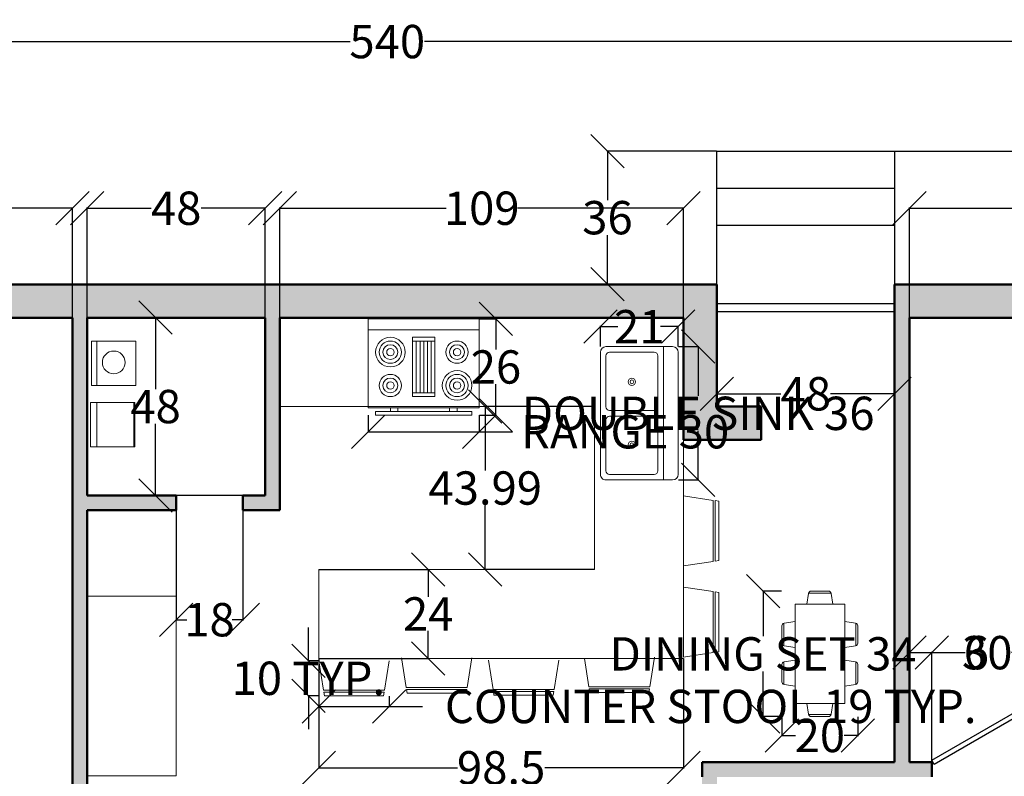
# Model space of a CAD drawing. Units: inches. Extents: x -9 to 615, y -420 to 89.
# Tile 5 of 6: x 201 to 467, y -115 to 89. Entities that reach past the tile are written whole.
import ezdxf

# ---------------------------------------------------------------- set-up
doc = ezdxf.new("R2010")
doc.units = ezdxf.units.IN
doc.header["$MEASUREMENT"] = 0
for name, color, linetype, lineweight in [('A-ANNO-DIMS', 2, 'Continuous', 18), ('A-DOOR', 4, 'Continuous', 25), ('A-EQPM', 8, 'Continuous', 18), ('A-FLOR-CASE', 32, 'Continuous', 18), ('A-FLOR-FIXT', 9, 'Continuous', 18), ('A-FLOR-STRS', 7, 'Continuous', 25), ('A-FURN', 8, 'Continuous', 18), ('A-WALL', 7, 'Continuous', 50)]:
    doc.layers.add(name, color=color, linetype=linetype, lineweight=lineweight)
doc.layers.add('A-WALL-PATT', color=251, linetype='Continuous', lineweight=13, true_color=0x636466)
doc.styles.get("Standard").update_dxf_attribs({"font": 'arial.ttf'})
doc.dimstyles.get("Standard").update_dxf_attribs({"dimtxt": 9, "dimasz": 9, "dimexe": 0.18, "dimexo": 0.0625, "dimgap": 0.09, "dimtad": 0, "dimtih": 1, "dimtoh": 1, "dimdec": 0, "dimzin": 0, "dimdsep": 46, "dimlunit": 4, "dimtxsty": 'Standard', "dimblk": 'OBLIQUE', "dimblk2": 'OBLIQUE', "dimcen": 0.09, "dimadec": 0, "dimazin": 0, "dimtfac": 1, "dimtdec": 0, "dimtofl": 0, "dimtmove": 0, "dimatfit": 3, "dimldrblk": 'OBLIQUE', "dimfxl": 1, "dimtolj": 1, "dimtzin": 0, "dimarcsym": 0})

# ---------------------------------------------------------------- blocks, each defined once
blk = doc.blocks.new('Range-Oven - 30 in top')
for p, q in [((0, -3), (30, -3)), ((12, -6), (18, -6)), ((13, -20), (13, -6)), ((14, -6), (14, -20)), ((15, -20), (15, -6)), ((16, -6), (16, -20)), ((17, -20), (17, -6)), ((18, -20), (12, -20)), ((6, -24), (6, -25)), ((8, -25), (8, -24)), ((22, -25), (22, -24)), ((24, -24), (24, -25))]:
    blk.add_line(p, q)
for points in [[(0, -24), (0, 0), (30, 0), (30, -24)], [(12, -21), (12, -5), (18, -5), (18, -21)], [(2, -26), (2, -25), (28, -25), (28, -26)]]:
    blk.add_lwpolyline(points, close=True)
for centre, radius in [((6, -9), 4), ((6, -9), 3), ((6, -9), 2), ((24, -9), 3), ((24, -9), 2), ((6, -9), 1), ((24, -9), 1), ((6, -18), 3), ((24, -18), 4), ((24, -18), 3), ((6, -18), 2), ((6, -18), 1), ((24, -18), 2), ((24, -18), 1)]:
    blk.add_circle(centre, radius)
blk = doc.blocks.new('Sink-double - 36 in top')
for p, q in [((-18, -4), (18, -4)), ((-0.75, -18.5), (-0.75, -6.5)), ((0.75, -6.5), (0.75, -18.5))]:
    blk.add_line(p, q)
for points in [[(-16.5, 0), (16.5, 0)], [(-18, -19.5), (-18, -1.5)], [(18, -1.5), (18, -19.5)], [(-16.5, -18.5), (-16.5, -6.5)], [(-15.5, -5.5), (-1.75, -5.5)], [(1.75, -5.5), (15.5, -5.5)], [(16.5, -6.5), (16.5, -18.5)], [(16.5, -21), (-16.5, -21)], [(-1.75, -19.5), (-15.5, -19.5)], [(15.5, -19.5), (1.75, -19.5)]]:
    blk.add_lwpolyline(points)
for centre, radius in [((-8.5, -12.5), 1), ((-8.5, -12.5), 0.5), ((8.5, -12.5), 1), ((8.5, -12.5), 0.5)]:
    blk.add_circle(centre, radius)
for centre, radius, start, end in [((-16.5, -1.5), 1.5, 90, 180), ((16.5, -1.5), 1.5, 0, 90), ((-15.5, -6.5), 1, 90, 180), ((-1.75, -6.5), 1, 0, 90), ((1.75, -6.5), 1, 90, 180), ((15.5, -6.5), 1, 0, 90), ((-15.5, -18.5), 1, 180, 270), ((-1.75, -18.5), 1, 270, 0), ((1.75, -18.5), 1, 180, 270), ((15.5, -18.5), 1, 270, 0), ((-16.5, -19.5), 1.5, 180, 270), ((16.5, -19.5), 1.5, 270, 0)]:
    blk.add_arc(centre, radius, start, end)
blk = doc.blocks.new('Dining Set - 36 x 72 in.')
for p, q in [((-22.26, 25.81), (-23.48, 18)), ((-22.23, 26), (-5.76, 26)), ((-20.29, 27.5), (-7.71, 27.5)), ((-4.52, 18), (-5.74, 25.81)), ((5.74, 25.81), (4.52, 18)), ((5.77, 26), (22.24, 26)), ((7.71, 27.5), (20.29, 27.5)), ((23.48, 18), (22.26, 25.81)), ((36, 18), (-36, 18)), ((-36, 18), (-36, -18)), ((36, -18), (36, 18)), ((-44, 8.23), (-44, -8.24)), ((-43.81, 8.26), (-36, 9.48)), ((43.81, 8.26), (36, 9.48)), ((44, 8.23), (44, -8.24)), ((-45.5, 6.29), (-45.5, -6.29)), ((45.5, 6.29), (45.5, -6.29)), ((-36, -9.48), (-43.81, -8.26)), ((36, -9.48), (43.81, -8.26)), ((-36, -18), (36, -18)), ((-22.26, -25.81), (-23.48, -18)), ((-4.52, -18), (-5.74, -25.81)), ((5.74, -25.81), (4.52, -18)), ((23.48, -18), (22.26, -25.81)), ((-22.23, -26), (-5.76, -26)), ((-20.29, -27.5), (-7.71, -27.5)), ((5.77, -26), (22.24, -26)), ((7.71, -27.5), (20.29, -27.5))]:
    blk.add_line(p, q)
for centre, start, end in [((-20.29, 25.5), 90, 171.11979), ((-7.71, 25.5), 8.88096, 90), ((7.71, 25.5), 90, 171.11979), ((20.29, 25.5), 8.88096, 90), ((-43.5, 6.29), 98.8806, 180), ((43.5, 6.29), 0, 81.1194), ((-43.5, -6.29), 180, 261.11938), ((43.5, -6.29), 278.88062, 0), ((-20.29, -25.5), 188.8802, 270), ((-7.71, -25.5), 270, 351.11906), ((7.71, -25.5), 188.8802, 270), ((20.29, -25.5), 270, 351.11906)]:
    blk.add_arc(centre, 2, start, end)
blk = doc.blocks.new('*U14')
for p, q in [((0, 0), (0, 6)), ((40, 0), (40, 6))]:
    blk.add_line(p, q)
blk.add_lwpolyline([(0, 0), (40, 0), (40, 1.75), (0, 1.75)], close=True)
blk = doc.blocks.new('*U12')
for p, q in [((0, 0), (0, -6)), ((40, 0), (40, -6))]:
    blk.add_line(p, q)
blk.add_lwpolyline([(0, 0), (34.64, 20), (35.52, 18.48), (0.87, -1.52)], close=True)
blk.add_arc((0, 0), 40, 0, 30)
blk = doc.blocks.new('CHAIR-COUNTER')
for p, q in [((8, 17.72), (0, 18.97)), ((8, 17.72), (8, 1.25)), ((9.5, 17.48), (8.5, 17.64)), ((8.5, 1.33), (8.5, 17.64)), ((9.5, 17.48), (9.5, 1.48)), ((0, 0), (8, 1.25)), ((8.5, 1.33), (9.5, 1.48))]:
    blk.add_line(p, q)
blk = doc.blocks.new('_Oblique')
at = {"color": 0, "linetype": 'ByBlock', "lineweight": -2}
blk.add_line((-0.5, -0.5), (0.5, 0.5), dxfattribs=at)
blk = doc.blocks.new('*D26')
at = {"layer": 'A-ANNO-DIMS', "color": 0, "lineweight": -2, "transparency": 16777216}
for p, q in [((281.97, -93.16), (281.97, -96.13)), ((300.94, -93.16), (300.94, -96.13)), ((281.97, -95.95), (300.94, -95.95)), ((300.94, -95.95), (309.94, -95.95))]:
    blk.add_line(p, q, dxfattribs=at)
at = {"layer": 'Defpoints', "color": 0, "transparency": 16777216}
for p in [(281.97, -93.1), (300.94, -93.1), (300.94, -95.95)]:
    blk.add_point(p, dxfattribs=at)
at = {"layer": 'A-ANNO-DIMS', "color": 0, "lineweight": -2, "transparency": 16777216, "xscale": 9, "yscale": 9, "zscale": 9, "rotation": 180}
blk.add_blockref('_Oblique', (281.97, -95.95), dxfattribs=at)
at = {"layer": 'A-ANNO-DIMS', "color": 0, "lineweight": -2, "transparency": 16777216, "xscale": 9, "yscale": 9, "zscale": 9}
blk.add_blockref('_Oblique', (300.94, -95.95), dxfattribs=at)
at = {"layer": 'A-ANNO-DIMS', "color": 0, "transparency": 16777216, "insert": (387.77, -95.95), "char_height": 9, "attachment_point": 5}
blk.add_mtext('\\A1;COUNTER STOOL 19 TYP.', dxfattribs=at)
blk = doc.blocks.new('*D27')
at = {"layer": 'A-ANNO-DIMS', "color": 0, "lineweight": -2, "transparency": 16777216}
for p, q in [((279.13, -83.6), (279.13, -74.6)), ((281.91, -83.6), (278.95, -83.6)), ((281.91, -93.1), (278.95, -93.1)), ((279.13, -93.1), (279.13, -102.1))]:
    blk.add_line(p, q, dxfattribs=at)
at = {"layer": 'Defpoints', "color": 0, "transparency": 16777216}
for p in [(281.97, -83.6), (279.13, -93.1), (281.97, -93.1)]:
    blk.add_point(p, dxfattribs=at)
at = {"layer": 'A-ANNO-DIMS', "color": 0, "lineweight": -2, "transparency": 16777216, "xscale": 9, "yscale": 9, "zscale": 9}
for p, rotation in [((279.13, -83.6), 270), ((279.13, -93.1), 90)]:
    blk.add_blockref('_Oblique', p, dxfattribs=dict(at, rotation=rotation))
at = {"layer": 'A-ANNO-DIMS', "color": 0, "transparency": 16777216, "insert": (279.13, -88.35), "char_height": 9, "attachment_point": 5}
blk.add_mtext('\\A1;10 TYP.', dxfattribs=at)
blk = doc.blocks.new('*D32')
at = {"layer": 'A-ANNO-DIMS', "color": 0, "lineweight": -2, "transparency": 16777216}
for p, q in [((295.28, -17.35), (295.28, -21.97)), ((325.28, -17.35), (325.28, -21.97)), ((295.28, -21.79), (325.28, -21.79)), ((325.28, -21.79), (334.28, -21.79))]:
    blk.add_line(p, q, dxfattribs=at)
at = {"layer": 'Defpoints', "color": 0, "transparency": 16777216}
for p in [(295.28, -17.29), (325.28, -17.29), (325.28, -21.79)]:
    blk.add_point(p, dxfattribs=at)
at = {"layer": 'A-ANNO-DIMS', "color": 0, "lineweight": -2, "transparency": 16777216, "xscale": 9, "yscale": 9, "zscale": 9, "rotation": 180}
blk.add_blockref('_Oblique', (295.28, -21.79), dxfattribs=at)
at = {"layer": 'A-ANNO-DIMS', "color": 0, "lineweight": -2, "transparency": 16777216, "xscale": 9, "yscale": 9, "zscale": 9}
blk.add_blockref('_Oblique', (325.28, -21.79), dxfattribs=at)
at = {"layer": 'A-ANNO-DIMS', "color": 0, "transparency": 16777216, "insert": (364.67, -21.79), "char_height": 9, "attachment_point": 5}
blk.add_mtext('\\A1;RANGE 30', dxfattribs=at)
blk = doc.blocks.new('*D33')
at = {"layer": 'A-ANNO-DIMS', "color": 0, "lineweight": -2, "transparency": 16777216}
for p, q in [((325.34, 8.71), (329.96, 8.71)), ((329.78, 8.71), (329.78, 0.4)), ((329.78, -17.29), (329.78, -8.97)), ((325.34, -17.29), (329.96, -17.29))]:
    blk.add_line(p, q, dxfattribs=at)
at = {"layer": 'Defpoints', "color": 0, "transparency": 16777216}
for p in [(325.28, 8.71), (329.78, 8.71), (325.28, -17.29)]:
    blk.add_point(p, dxfattribs=at)
at = {"layer": 'A-ANNO-DIMS', "color": 0, "lineweight": -2, "transparency": 16777216, "xscale": 9, "yscale": 9, "zscale": 9}
for p, rotation in [((329.78, 8.71), 90), ((329.78, -17.29), 270)]:
    blk.add_blockref('_Oblique', p, dxfattribs=dict(at, rotation=rotation))
at = {"layer": 'A-ANNO-DIMS', "color": 0, "transparency": 16777216, "insert": (329.78, -4.29), "char_height": 9, "attachment_point": 5}
blk.add_mtext('\\A1;26', dxfattribs=at)
blk = doc.blocks.new('*D34')
at = {"layer": 'A-ANNO-DIMS', "color": 0, "lineweight": -2, "transparency": 16777216}
for p, q in [((379.05, 1.19), (384.57, 1.19)), ((384.39, 1.19), (384.39, -12.06)), ((384.39, -34.81), (384.39, -21.56)), ((379.05, -34.81), (384.57, -34.81))]:
    blk.add_line(p, q, dxfattribs=at)
at = {"layer": 'Defpoints', "color": 0, "transparency": 16777216}
for p in [(378.99, 1.19), (378.99, -34.81), (384.39, -34.81)]:
    blk.add_point(p, dxfattribs=at)
at = {"layer": 'A-ANNO-DIMS', "color": 0, "lineweight": -2, "transparency": 16777216, "xscale": 9, "yscale": 9, "zscale": 9}
for p, rotation in [((384.39, 1.19), 90), ((384.39, -34.81), 270)]:
    blk.add_blockref('_Oblique', p, dxfattribs=dict(at, rotation=rotation))
at = {"layer": 'A-ANNO-DIMS', "color": 0, "transparency": 16777216, "insert": (384.39, -16.81), "char_height": 9, "attachment_point": 5}
blk.add_mtext('\\A1;DOUBLE SINK 36', dxfattribs=at)
blk = doc.blocks.new('*D35')
at = {"layer": 'A-ANNO-DIMS', "color": 0, "lineweight": -2, "transparency": 16777216}
for p, q in [((357.99, 1.25), (357.99, 6.77)), ((357.99, 6.59), (362.74, 6.59)), ((378.99, 6.59), (374.23, 6.59)), ((378.99, 1.25), (378.99, 6.77))]:
    blk.add_line(p, q, dxfattribs=at)
at = {"layer": 'Defpoints', "color": 0, "transparency": 16777216}
for p in [(378.99, 6.59), (357.99, 1.19), (378.99, 1.19)]:
    blk.add_point(p, dxfattribs=at)
at = {"layer": 'A-ANNO-DIMS', "color": 0, "lineweight": -2, "transparency": 16777216, "xscale": 9, "yscale": 9, "zscale": 9, "rotation": 180}
blk.add_blockref('_Oblique', (357.99, 6.59), dxfattribs=at)
at = {"layer": 'A-ANNO-DIMS', "color": 0, "lineweight": -2, "transparency": 16777216, "xscale": 9, "yscale": 9, "zscale": 9}
blk.add_blockref('_Oblique', (378.99, 6.59), dxfattribs=at)
at = {"layer": 'A-ANNO-DIMS', "color": 0, "transparency": 16777216, "insert": (368.49, 6.59), "char_height": 9, "attachment_point": 5}
blk.add_mtext('\\A1;21', dxfattribs=at)
blk = doc.blocks.new('*D38')
at = {"layer": 'A-ANNO-DIMS', "color": 0, "lineweight": -2, "transparency": 16777216}
for p, q in [((406.93, -64.79), (401.73, -64.79)), ((401.91, -64.79), (401.91, -77)), ((401.91, -98.71), (401.91, -86.5)), ((406.93, -98.71), (401.73, -98.71))]:
    blk.add_line(p, q, dxfattribs=at)
at = {"layer": 'Defpoints', "color": 0, "transparency": 16777216}
for p in [(407, -64.79), (401.91, -98.71), (407, -98.71)]:
    blk.add_point(p, dxfattribs=at)
at = {"layer": 'A-ANNO-DIMS', "color": 0, "lineweight": -2, "transparency": 16777216, "xscale": 9, "yscale": 9, "zscale": 9}
for p, rotation in [((401.91, -64.79), 90), ((401.91, -98.71), 270)]:
    blk.add_blockref('_Oblique', p, dxfattribs=dict(at, rotation=rotation))
at = {"layer": 'A-ANNO-DIMS', "color": 0, "transparency": 16777216, "insert": (401.91, -81.75), "char_height": 9, "attachment_point": 5}
blk.add_mtext('\\A1;DINING SET 34', dxfattribs=at)
blk = doc.blocks.new('*D39')
at = {"layer": 'A-ANNO-DIMS', "color": 0, "lineweight": -2, "transparency": 16777216}
for p, q in [((407, -98.77), (407, -103.97)), ((427.49, -98.77), (427.49, -103.97)), ((407, -103.79), (410.65, -103.79)), ((427.49, -103.79), (423.84, -103.79))]:
    blk.add_line(p, q, dxfattribs=at)
at = {"layer": 'Defpoints', "color": 0, "transparency": 16777216}
for p in [(407, -98.71), (427.49, -98.71), (427.49, -103.79)]:
    blk.add_point(p, dxfattribs=at)
at = {"layer": 'A-ANNO-DIMS', "color": 0, "lineweight": -2, "transparency": 16777216, "xscale": 9, "yscale": 9, "zscale": 9, "rotation": 180}
blk.add_blockref('_Oblique', (407, -103.79), dxfattribs=at)
at = {"layer": 'A-ANNO-DIMS', "color": 0, "lineweight": -2, "transparency": 16777216, "xscale": 9, "yscale": 9, "zscale": 9}
blk.add_blockref('_Oblique', (427.49, -103.79), dxfattribs=at)
at = {"layer": 'A-ANNO-DIMS', "color": 0, "transparency": 16777216, "insert": (417.24, -103.79), "char_height": 9, "attachment_point": 5}
blk.add_mtext('\\A1;20', dxfattribs=at)
blk = doc.blocks.new('*D40')
at = {"layer": 'A-ANNO-DIMS', "color": 0, "lineweight": -2, "transparency": 16777216}
for p, q in [((30.44, 18.08), (30.44, 83.75)), ((30.44, 83.57), (290.42, 83.57)), ((570.44, 83.57), (310.45, 83.57)), ((570.44, 18.08), (570.44, 83.75))]:
    blk.add_line(p, q, dxfattribs=at)
at = {"layer": 'Defpoints', "color": 0, "transparency": 16777216}
for p in [(570.44, 83.57), (30.44, 18.02), (570.44, 18.02)]:
    blk.add_point(p, dxfattribs=at)
at = {"layer": 'A-ANNO-DIMS', "color": 0, "lineweight": -2, "transparency": 16777216, "xscale": 9, "yscale": 9, "zscale": 9, "rotation": 180}
blk.add_blockref('_Oblique', (30.44, 83.57), dxfattribs=at)
at = {"layer": 'A-ANNO-DIMS', "color": 0, "lineweight": -2, "transparency": 16777216, "xscale": 9, "yscale": 9, "zscale": 9}
blk.add_blockref('_Oblique', (570.44, 83.57), dxfattribs=at)
at = {"layer": 'A-ANNO-DIMS', "color": 0, "transparency": 16777216, "insert": (300.44, 83.57), "char_height": 9, "attachment_point": 5}
blk.add_mtext('\\A1;540', dxfattribs=at)
blk = doc.blocks.new('*D42')
at = {"layer": 'A-ANNO-DIMS', "color": 0, "lineweight": -2, "transparency": 16777216}
for p, q in [((437.5, 54.02), (600.17, 54.02)), ((599.99, 54.02), (599.99, -160.45)), ((599.99, -384.29), (599.99, -169.82)), ((365.62, -384.29), (600.17, -384.29))]:
    blk.add_line(p, q, dxfattribs=at)
at = {"layer": 'Defpoints', "color": 0, "transparency": 16777216}
for p in [(437.44, 54.02), (599.99, 54.02), (365.56, -384.29)]:
    blk.add_point(p, dxfattribs=at)
at = {"layer": 'A-ANNO-DIMS', "color": 0, "lineweight": -2, "transparency": 16777216, "xscale": 9, "yscale": 9, "zscale": 9}
for p, rotation in [((599.99, 54.02), 90), ((599.99, -384.29), 270)]:
    blk.add_blockref('_Oblique', p, dxfattribs=dict(at, rotation=rotation))
at = {"layer": 'A-ANNO-DIMS', "color": 0, "transparency": 16777216, "insert": (599.99, -165.14), "char_height": 9, "attachment_point": 5}
blk.add_mtext('\\A1;438.3', dxfattribs=at)
blk = doc.blocks.new('*D43')
at = {"layer": 'A-ANNO-DIMS', "color": 0, "lineweight": -2, "transparency": 16777216}
for p, q in [((39.44, 9.08), (39.44, 38.75)), ((39.44, 38.57), (117.83, 38.57)), ((215.44, 38.57), (137.04, 38.57)), ((215.44, 9.08), (215.44, 38.75))]:
    blk.add_line(p, q, dxfattribs=at)
at = {"layer": 'Defpoints', "color": 0, "transparency": 16777216}
for p in [(215.44, 38.57), (39.44, 9.02), (215.44, 9.02)]:
    blk.add_point(p, dxfattribs=at)
at = {"layer": 'A-ANNO-DIMS', "color": 0, "lineweight": -2, "transparency": 16777216, "xscale": 9, "yscale": 9, "zscale": 9, "rotation": 180}
blk.add_blockref('_Oblique', (39.44, 38.57), dxfattribs=at)
at = {"layer": 'A-ANNO-DIMS', "color": 0, "lineweight": -2, "transparency": 16777216, "xscale": 9, "yscale": 9, "zscale": 9}
blk.add_blockref('_Oblique', (215.44, 38.57), dxfattribs=at)
at = {"layer": 'A-ANNO-DIMS', "color": 0, "transparency": 16777216, "insert": (127.44, 38.57), "char_height": 9, "attachment_point": 5}
blk.add_mtext('\\A1;176', dxfattribs=at)
blk = doc.blocks.new('*D44')
at = {"layer": 'A-ANNO-DIMS', "color": 0, "lineweight": -2, "transparency": 16777216}
for p, q in [((219.44, 9.08), (219.44, 38.75)), ((219.44, 38.57), (236.71, 38.57)), ((267.44, 38.57), (250.16, 38.57)), ((267.44, 9.08), (267.44, 38.75))]:
    blk.add_line(p, q, dxfattribs=at)
at = {"layer": 'Defpoints', "color": 0, "transparency": 16777216}
for p in [(267.44, 38.57), (219.44, 9.02), (267.44, 9.02)]:
    blk.add_point(p, dxfattribs=at)
at = {"layer": 'A-ANNO-DIMS', "color": 0, "lineweight": -2, "transparency": 16777216, "xscale": 9, "yscale": 9, "zscale": 9, "rotation": 180}
blk.add_blockref('_Oblique', (219.44, 38.57), dxfattribs=at)
at = {"layer": 'A-ANNO-DIMS', "color": 0, "lineweight": -2, "transparency": 16777216, "xscale": 9, "yscale": 9, "zscale": 9}
blk.add_blockref('_Oblique', (267.44, 38.57), dxfattribs=at)
at = {"layer": 'A-ANNO-DIMS', "color": 0, "transparency": 16777216, "insert": (243.44, 38.57), "char_height": 9, "attachment_point": 5}
blk.add_mtext('\\A1;48', dxfattribs=at)
blk = doc.blocks.new('*D45')
at = {"layer": 'A-ANNO-DIMS', "color": 0, "lineweight": -2, "transparency": 16777216}
for p, q in [((271.44, 9.08), (271.44, 38.75)), ((271.44, 38.57), (316.32, 38.57)), ((380.44, 38.57), (335.56, 38.57)), ((380.44, 9.08), (380.44, 38.75))]:
    blk.add_line(p, q, dxfattribs=at)
at = {"layer": 'Defpoints', "color": 0, "transparency": 16777216}
for p in [(380.44, 38.57), (271.44, 9.02), (380.44, 9.02)]:
    blk.add_point(p, dxfattribs=at)
at = {"layer": 'A-ANNO-DIMS', "color": 0, "lineweight": -2, "transparency": 16777216, "xscale": 9, "yscale": 9, "zscale": 9, "rotation": 180}
blk.add_blockref('_Oblique', (271.44, 38.57), dxfattribs=at)
at = {"layer": 'A-ANNO-DIMS', "color": 0, "lineweight": -2, "transparency": 16777216, "xscale": 9, "yscale": 9, "zscale": 9}
blk.add_blockref('_Oblique', (380.44, 38.57), dxfattribs=at)
at = {"layer": 'A-ANNO-DIMS', "color": 0, "transparency": 16777216, "insert": (325.94, 38.57), "char_height": 9, "attachment_point": 5}
blk.add_mtext('\\A1;109', dxfattribs=at)
blk = doc.blocks.new('*D46')
at = {"layer": 'A-ANNO-DIMS', "color": 0, "lineweight": -2, "transparency": 16777216}
for p, q in [((389.44, 17.96), (389.44, -11.71)), ((437.44, 17.96), (437.44, -11.71)), ((389.44, -11.53), (406.71, -11.53)), ((437.44, -11.53), (420.16, -11.53))]:
    blk.add_line(p, q, dxfattribs=at)
at = {"layer": 'Defpoints', "color": 0, "transparency": 16777216}
for p in [(389.44, 18.02), (437.44, 18.02), (389.44, -11.53)]:
    blk.add_point(p, dxfattribs=at)
at = {"layer": 'A-ANNO-DIMS', "color": 0, "lineweight": -2, "transparency": 16777216, "xscale": 9, "yscale": 9, "zscale": 9, "rotation": 180}
blk.add_blockref('_Oblique', (389.44, -11.53), dxfattribs=at)
at = {"layer": 'A-ANNO-DIMS', "color": 0, "lineweight": -2, "transparency": 16777216, "xscale": 9, "yscale": 9, "zscale": 9}
blk.add_blockref('_Oblique', (437.44, -11.53), dxfattribs=at)
at = {"layer": 'A-ANNO-DIMS', "color": 0, "transparency": 16777216, "insert": (413.44, -11.53), "char_height": 9, "attachment_point": 5}
blk.add_mtext('\\A1;48', dxfattribs=at)
blk = doc.blocks.new('*D47')
at = {"layer": 'A-ANNO-DIMS', "color": 0, "lineweight": -2, "transparency": 16777216}
for p, q in [((441.44, 9.08), (441.44, 38.75)), ((441.44, 38.57), (491.84, 38.57)), ((561.44, 38.57), (511.03, 38.57)), ((561.44, 9.08), (561.44, 38.75))]:
    blk.add_line(p, q, dxfattribs=at)
at = {"layer": 'Defpoints', "color": 0, "transparency": 16777216}
for p in [(561.44, 38.57), (441.44, 9.02), (561.44, 9.02)]:
    blk.add_point(p, dxfattribs=at)
at = {"layer": 'A-ANNO-DIMS', "color": 0, "lineweight": -2, "transparency": 16777216, "xscale": 9, "yscale": 9, "zscale": 9, "rotation": 180}
blk.add_blockref('_Oblique', (441.44, 38.57), dxfattribs=at)
at = {"layer": 'A-ANNO-DIMS', "color": 0, "lineweight": -2, "transparency": 16777216, "xscale": 9, "yscale": 9, "zscale": 9}
blk.add_blockref('_Oblique', (561.44, 38.57), dxfattribs=at)
at = {"layer": 'A-ANNO-DIMS', "color": 0, "transparency": 16777216, "insert": (501.44, 38.57), "char_height": 9, "attachment_point": 5}
blk.add_mtext('\\A1;120', dxfattribs=at)
blk = doc.blocks.new('*D48')
at = {"layer": 'A-ANNO-DIMS', "color": 0, "lineweight": -2, "transparency": 16777216}
for p, q in [((389.38, 54.02), (359.71, 54.02)), ((359.89, 54.02), (359.89, 40.71)), ((359.89, 18.02), (359.89, 31.33)), ((389.38, 18.02), (359.71, 18.02))]:
    blk.add_line(p, q, dxfattribs=at)
at = {"layer": 'Defpoints', "color": 0, "transparency": 16777216}
for p in [(359.89, 54.02), (389.44, 54.02), (389.44, 18.02)]:
    blk.add_point(p, dxfattribs=at)
at = {"layer": 'A-ANNO-DIMS', "color": 0, "lineweight": -2, "transparency": 16777216, "xscale": 9, "yscale": 9, "zscale": 9}
for p, rotation in [((359.89, 54.02), 90), ((359.89, 18.02), 270)]:
    blk.add_blockref('_Oblique', p, dxfattribs=dict(at, rotation=rotation))
at = {"layer": 'A-ANNO-DIMS', "color": 0, "transparency": 16777216, "insert": (359.89, 36.02), "char_height": 9, "attachment_point": 5}
blk.add_mtext('\\A1;36', dxfattribs=at)
blk = doc.blocks.new('*D64')
at = {"layer": 'A-ANNO-DIMS', "color": 0, "lineweight": -2, "transparency": 16777216}
for p, q in [((267.38, 9.02), (237.71, 9.02)), ((237.89, 9.02), (237.89, -10.3)), ((237.89, -38.98), (237.89, -19.67)), ((267.38, -38.98), (237.71, -38.98))]:
    blk.add_line(p, q, dxfattribs=at)
at = {"layer": 'Defpoints', "color": 0, "transparency": 16777216}
for p in [(237.89, 9.02), (267.44, 9.02), (267.44, -38.98)]:
    blk.add_point(p, dxfattribs=at)
at = {"layer": 'A-ANNO-DIMS', "color": 0, "lineweight": -2, "transparency": 16777216, "xscale": 9, "yscale": 9, "zscale": 9}
for p, rotation in [((237.89, 9.02), 90), ((237.89, -38.98), 270)]:
    blk.add_blockref('_Oblique', p, dxfattribs=dict(at, rotation=rotation))
at = {"layer": 'A-ANNO-DIMS', "color": 0, "transparency": 16777216, "insert": (237.89, -14.98), "char_height": 9, "attachment_point": 5}
blk.add_mtext('\\A1;48', dxfattribs=at)
blk = doc.blocks.new('*D69')
at = {"layer": 'A-ANNO-DIMS', "color": 0, "lineweight": -2, "transparency": 16777216}
for p, q in [((281.94, -83.03), (281.94, -112.7)), ((380.44, -83.03), (380.44, -112.7)), ((281.94, -112.52), (319.37, -112.52)), ((380.44, -112.52), (343, -112.52))]:
    blk.add_line(p, q, dxfattribs=at)
at = {"layer": 'Defpoints', "color": 0, "transparency": 16777216}
for p in [(281.94, -82.97), (380.44, -82.97), (281.94, -112.52)]:
    blk.add_point(p, dxfattribs=at)
at = {"layer": 'A-ANNO-DIMS', "color": 0, "lineweight": -2, "transparency": 16777216, "xscale": 9, "yscale": 9, "zscale": 9, "rotation": 180}
blk.add_blockref('_Oblique', (281.94, -112.52), dxfattribs=at)
at = {"layer": 'A-ANNO-DIMS', "color": 0, "lineweight": -2, "transparency": 16777216, "xscale": 9, "yscale": 9, "zscale": 9}
blk.add_blockref('_Oblique', (380.44, -112.52), dxfattribs=at)
at = {"layer": 'A-ANNO-DIMS', "color": 0, "transparency": 16777216, "insert": (331.19, -112.52), "char_height": 9, "attachment_point": 5}
blk.add_mtext('\\A1;98.5', dxfattribs=at)
blk = doc.blocks.new('*D70')
at = {"layer": 'A-ANNO-DIMS', "color": 0, "lineweight": -2, "transparency": 16777216}
for p, q in [((356.38, -14.98), (326.71, -14.98)), ((326.89, -14.98), (326.89, -32.29)), ((326.89, -58.97), (326.89, -41.66)), ((356.38, -58.97), (326.71, -58.97))]:
    blk.add_line(p, q, dxfattribs=at)
at = {"layer": 'Defpoints', "color": 0, "transparency": 16777216}
for p in [(326.89, -14.98), (356.44, -14.98), (356.44, -58.97)]:
    blk.add_point(p, dxfattribs=at)
at = {"layer": 'A-ANNO-DIMS', "color": 0, "lineweight": -2, "transparency": 16777216, "xscale": 9, "yscale": 9, "zscale": 9}
for p, rotation in [((326.89, -14.98), 90), ((326.89, -58.97), 270)]:
    blk.add_blockref('_Oblique', p, dxfattribs=dict(at, rotation=rotation))
at = {"layer": 'A-ANNO-DIMS', "color": 0, "transparency": 16777216, "insert": (326.89, -36.98), "char_height": 9, "attachment_point": 5}
blk.add_mtext('\\A1;43.99', dxfattribs=at)
blk = doc.blocks.new('*D71')
at = {"layer": 'A-ANNO-DIMS', "color": 0, "lineweight": -2, "transparency": 16777216}
for p, q in [((282, -58.97), (311.67, -58.97)), ((311.49, -58.97), (311.49, -66.36)), ((311.49, -82.97), (311.49, -75.58)), ((282, -82.97), (311.67, -82.97))]:
    blk.add_line(p, q, dxfattribs=at)
at = {"layer": 'Defpoints', "color": 0, "transparency": 16777216}
for p in [(281.94, -58.97), (281.94, -82.97), (311.49, -82.97)]:
    blk.add_point(p, dxfattribs=at)
at = {"layer": 'A-ANNO-DIMS', "color": 0, "lineweight": -2, "transparency": 16777216, "xscale": 9, "yscale": 9, "zscale": 9}
for p, rotation in [((311.49, -58.97), 90), ((311.49, -82.97), 270)]:
    blk.add_blockref('_Oblique', p, dxfattribs=dict(at, rotation=rotation))
at = {"layer": 'A-ANNO-DIMS', "color": 0, "transparency": 16777216, "insert": (311.49, -70.97), "char_height": 9, "attachment_point": 5}
blk.add_mtext('\\A1;24', dxfattribs=at)
blk = doc.blocks.new('*D81')
at = {"layer": 'A-ANNO-DIMS', "color": 0, "lineweight": -2, "transparency": 16777216}
for p, q in [((441.44, -110.92), (441.44, -81.25)), ((441.44, -81.43), (447.44, -81.43)), ((447.44, -110.92), (447.44, -81.25)), ((447.44, -81.43), (456.44, -81.43))]:
    blk.add_line(p, q, dxfattribs=at)
at = {"layer": 'Defpoints', "color": 0, "transparency": 16777216}
for p in [(447.44, -81.43), (441.44, -110.98), (447.44, -110.98)]:
    blk.add_point(p, dxfattribs=at)
at = {"layer": 'A-ANNO-DIMS', "color": 0, "lineweight": -2, "transparency": 16777216, "xscale": 9, "yscale": 9, "zscale": 9, "rotation": 180}
blk.add_blockref('_Oblique', (441.44, -81.43), dxfattribs=at)
at = {"layer": 'A-ANNO-DIMS', "color": 0, "lineweight": -2, "transparency": 16777216, "xscale": 9, "yscale": 9, "zscale": 9}
blk.add_blockref('_Oblique', (447.44, -81.43), dxfattribs=at)
at = {"layer": 'A-ANNO-DIMS', "color": 0, "transparency": 16777216, "insert": (459.5, -81.43), "char_height": 9, "attachment_point": 5}
blk.add_mtext('\\A1;6', dxfattribs=at)
blk = doc.blocks.new('*D82')
at = {"layer": 'A-ANNO-DIMS', "color": 0, "lineweight": -2, "transparency": 16777216}
for p, q in [((447.44, -110.92), (447.44, -81.25)), ((447.44, -81.43), (455.92, -81.43)), ((477.44, -81.43), (468.96, -81.43)), ((477.44, -110.92), (477.44, -81.25))]:
    blk.add_line(p, q, dxfattribs=at)
at = {"layer": 'Defpoints', "color": 0, "transparency": 16777216}
for p in [(477.44, -81.43), (447.44, -110.98), (477.44, -110.98)]:
    blk.add_point(p, dxfattribs=at)
at = {"layer": 'A-ANNO-DIMS', "color": 0, "lineweight": -2, "transparency": 16777216, "xscale": 9, "yscale": 9, "zscale": 9, "rotation": 180}
blk.add_blockref('_Oblique', (447.44, -81.43), dxfattribs=at)
at = {"layer": 'A-ANNO-DIMS', "color": 0, "lineweight": -2, "transparency": 16777216, "xscale": 9, "yscale": 9, "zscale": 9}
blk.add_blockref('_Oblique', (477.44, -81.43), dxfattribs=at)
at = {"layer": 'A-ANNO-DIMS', "color": 0, "transparency": 16777216, "insert": (462.44, -81.43), "char_height": 9, "attachment_point": 5}
blk.add_mtext('\\A1;30', dxfattribs=at)
blk = doc.blocks.new('*D89')
at = {"layer": 'A-ANNO-DIMS', "color": 0, "lineweight": -2, "transparency": 16777216}
for p, q in [((243.44, -43.04), (243.44, -72.71)), ((261.44, -43.04), (261.44, -72.71)), ((243.44, -72.53), (246.32, -72.53)), ((261.44, -72.53), (258.56, -72.53))]:
    blk.add_line(p, q, dxfattribs=at)
at = {"layer": 'Defpoints', "color": 0, "transparency": 16777216}
for p in [(243.44, -42.98), (261.44, -42.98), (243.44, -72.53)]:
    blk.add_point(p, dxfattribs=at)
at = {"layer": 'A-ANNO-DIMS', "color": 0, "lineweight": -2, "transparency": 16777216, "xscale": 9, "yscale": 9, "zscale": 9, "rotation": 180}
blk.add_blockref('_Oblique', (243.44, -72.53), dxfattribs=at)
at = {"layer": 'A-ANNO-DIMS', "color": 0, "lineweight": -2, "transparency": 16777216, "xscale": 9, "yscale": 9, "zscale": 9}
blk.add_blockref('_Oblique', (261.44, -72.53), dxfattribs=at)
at = {"layer": 'A-ANNO-DIMS', "color": 0, "transparency": 16777216, "insert": (252.44, -72.53), "char_height": 9, "attachment_point": 5}
blk.add_mtext('\\A1;18', dxfattribs=at)

msp = doc.modelspace()

# ---------------------------------------------------------------- hatches: boundary and pattern name
at = {"layer": 'A-WALL-PATT'}
h = msp.add_hatch(color=256, dxfattribs=at)
h.dxf.hatch_style = 1
h.paths.add_polyline_path([(389.4378, 18.0183), (30.4378, 18.0183), (30.4378, -341.9817), (316.4378, -341.9817), (316.4378, -336.5817), (316.4378, -332.9817), (283.4378, -332.9817), (283.4378, -256.9817), (283.4378, -250.9817), (283.4378, -248.9817), (278.9378, -248.9817), (277.4378, -248.9817), (277.4378, -250.9817), (277.4378, -256.9817), (211.4378, -256.9817), (211.4378, -260.9817), (279.4378, -260.9817), (279.4378, -332.9817), (175.4378, -332.9817), (175.4378, -260.9817), (181.4378, -260.9817), (181.4378, -256.9817), (175.4378, -256.9817), (175.4378, -248.9817), (171.4378, -248.9817), (171.4378, -332.9817), (39.4378, -332.9817), (39.4378, -212.9817), (171.4378, -212.9817), (171.4378, -218.9817), (175.4378, -218.9817), (175.4378, -212.9817), (179.4378, -212.9817), (179.4378, -208.9817), (135.4378, -208.9817), (135.4378, -114.9817), (179.4378, -114.9817), (179.4378, -110.9817), (100.4378, -110.9817), (100.4378, -114.9817), (131.4378, -114.9817), (131.4378, -208.9817), (39.4378, -208.9817), (39.4378, -114.9817), (70.4378, -114.9817), (70.4378, -110.9817), (39.4378, -110.9817), (39.4378, 9.0183), (215.4378, 9.0183), (215.4378, -110.9817), (215.4378, -208.9817), (209.4378, -208.9817), (209.4378, -212.9817), (215.4378, -212.9817), (255.4378, -212.9817), (277.4378, -212.9817), (277.4378, -218.9817), (283.4378, -218.9817), (283.4378, -212.9817), (283.4378, -208.9817), (283.4378, -202.9817), (279.4378, -202.9817), (279.4378, -208.9817), (255.4378, -208.9817), (219.4378, -208.9817), (219.4378, -170.1983), (255.4378, -170.1983), (277.4378, -170.1983), (277.4378, -176.1983), (283.4378, -176.1983), (283.4378, -170.1983), (283.4378, -166.1983), (255.4378, -166.1983), (219.4378, -166.1983), (219.4378, -42.9817), (243.4378, -42.9817), (243.4378, -38.9817), (219.4378, -38.9817), (219.4378, 9.0183), (267.4378, 9.0183), (267.4378, -38.9817), (261.4378, -38.9817), (261.4378, -42.9817), (271.4378, -42.9817), (271.4378, 9.0183), (380.4378, 9.0183), (380.4378, -14.9817), (380.4378, -23.9817), (401.4378, -23.9817), (401.4378, -14.9817), (389.4378, -14.9817)])
h = msp.add_hatch(color=256, dxfattribs=at)
h.dxf.hatch_style = 1
h.paths.add_polyline_path([(570.4378, 18.0183), (437.4378, 18.0183), (437.4378, -14.9817), (437.4378, -110.9817), (385.4378, -110.9817), (385.4378, -114.9817), (385.4378, -120.9817), (389.4378, -120.9817), (389.4378, -114.9817), (437.4378, -114.9817), (447.4378, -114.9817), (447.4378, -110.9817), (441.4378, -110.9817), (441.4378, 9.0183), (561.4378, 9.0183), (561.4378, -110.9817), (477.4378, -110.9817), (477.4378, -114.9817), (497.4378, -114.9817), (497.4378, -168.9817), (501.4378, -168.9817), (501.4378, -114.9817), (561.4378, -114.9817), (561.4378, -198.9817), (531.4378, -198.9817), (501.4378, -198.9817), (501.4378, -192.9817), (497.4378, -192.9817), (497.4378, -198.9817), (477.4378, -198.9817), (477.4378, -202.9817), (561.4378, -202.9817), (561.4378, -332.9817), (441.4378, -332.9817), (441.4378, -202.9817), (447.4378, -202.9817), (447.4378, -198.9817), (437.4378, -198.9817), (431.4378, -198.9817), (431.4378, -202.9817), (437.4378, -202.9817), (437.4378, -256.9817), (389.4378, -256.9817), (389.4378, -202.9799), (407.5704, -202.9799), (407.4511, -198.9817), (389.4378, -198.9817), (385.4378, -198.9817), (385.4378, -302.9817), (389.4378, -302.9817), (389.4378, -260.9817), (437.4378, -260.9817), (437.4378, -332.9817), (389.4378, -332.9817), (389.4378, -326.9817), (385.4378, -326.9817), (385.4378, -332.9817), (352.4378, -332.9817), (352.4378, -341.9817), (570.4378, -341.9817)])

# ---------------------------------------------------------------- linework, layer by layer
at = {"layer": 'A-EQPM'}
for p, q in [((221.9973, 2.7027), (221.9973, -9.2973)), ((222.0477, -13.8957), (222.0477, -25.8957)), ((231.9831, -13.8957), (231.9831, -25.8957))]:
    msp.add_line(p, q, dxfattribs=at)
for points in [[(220.5548, 2.7027), (232.5548, 2.7027), (232.5548, -9.2973), (220.5548, -9.2973)], [(220.3147, -13.8957), (232.3147, -13.8957), (232.3147, -25.8957), (220.3147, -25.8957)]]:
    msp.add_lwpolyline(points, close=True, dxfattribs=at)
msp.add_circle((226.5871, -3.0612), 3.0669, dxfattribs=at)
at = {"layer": 'A-FLOR-CASE'}
for p, q in [((271.4378, -14.9817), (356.4378, -14.9817)), ((356.4378, -14.9817), (356.4378, -58.9697)), ((380.4378, -23.9817), (380.4378, -82.6771)), ((243.4378, -114.6494), (243.4378, -42.9817)), ((356.4378, -58.9697), (281.9364, -58.9697)), ((281.9364, -58.9697), (281.9364, -82.9697)), ((243.4378, -66.1655), (219.4378, -66.1655)), ((356.4378, -82.9697), (281.9364, -82.9697)), ((356.4378, -82.9697), (380.4378, -82.9697)), ((243.4378, -114.6494), (219.4378, -114.6494))]:
    msp.add_line(p, q, dxfattribs=at)
at = {"layer": 'A-FLOR-STRS'}
for p, q in [((389.4378, 18.0183), (389.4378, 54.0183)), ((389.4378, 54.0183), (437.4378, 54.0183)), ((437.4378, 54.0183), (437.4378, 18.0183)), ((389.4378, 44.0183), (437.4378, 44.0183)), ((389.4378, 34.0183), (437.4378, 34.0183))]:
    msp.add_line(p, q, dxfattribs=at)
at = {"layer": 'A-FURN'}
for p, q in [((353.6503, -82.9697), (354.8549, -90.6788)), ((371.3237, -90.6801), (372.5741, -82.6771)), ((371.3198, -90.6795), (354.8502, -90.6795)), ((354.931, -91.1795), (371.2428, -91.1795)), ((354.9331, -91.1792), (355.0894, -92.1795)), ((371.0894, -92.1795), (355.0894, -92.1795)), ((371.0894, -92.1795), (371.2456, -91.18))]:
    msp.add_line(p, q, dxfattribs=at)
at = {"layer": 'A-WALL'}
for p, q in [((389.4378, -14.9817), (389.4378, 18.0183)), ((437.4378, 18.0183), (437.4378, -14.9817)), ((39.4378, 9.0183), (215.4378, 9.0183)), ((215.4378, -110.9817), (215.4378, 9.0183)), ((215.4378, -208.9817), (215.4378, 9.0183)), ((219.4378, 9.0183), (267.4378, 9.0183)), ((219.4378, -38.9817), (219.4378, 9.0183)), ((267.4378, -38.9817), (267.4378, 9.0183)), ((271.4378, -42.9817), (271.4378, 9.0183)), ((271.4378, 9.0183), (380.4378, 9.0183)), ((380.4378, -14.9817), (380.4378, 9.0183)), ((437.4378, 9.0183), (437.4378, -110.9817)), ((441.4378, 9.0183), (441.4378, -110.9817)), ((441.4378, 9.0183), (561.4378, 9.0183)), ((380.4378, -14.9817), (380.4378, -23.9817)), ((401.4378, -14.9817), (389.4378, -14.9817)), ((401.4378, -14.9817), (401.4378, -23.9817)), ((401.4378, -23.9817), (380.4378, -23.9817)), ((219.4378, -38.9817), (243.4378, -38.9817)), ((243.4378, -38.9817), (243.4378, -42.9817)), ((261.4378, -38.9817), (261.4378, -42.9817)), ((261.4378, -38.9817), (267.4378, -38.9817)), ((219.4378, -42.9817), (243.4378, -42.9817)), ((219.4378, -166.1983), (219.4378, -42.9817)), ((261.4378, -42.9817), (271.4378, -42.9817)), ((437.4378, -110.9817), (385.4378, -110.9817)), ((385.4378, -110.9817), (385.4378, -114.9817)), ((441.4378, -110.9817), (447.4378, -110.9817)), ((447.4378, -110.9817), (447.4378, -114.9817))]:
    msp.add_line(p, q, dxfattribs=at)
for points in [[(316.4378, -341.9817), (30.4378, -341.9817), (30.4378, 18.0183), (389.4378, 18.0183)], [(437.4378, 18.0183), (570.4378, 18.0183), (570.4378, -341.9817), (352.4378, -341.9817)]]:
    msp.add_lwpolyline(points, dxfattribs=at)

# ---------------------------------------------------------------- block references
at = {"layer": 'A-DOOR'}
for name, p, xscale, yscale, zscale in [('*U14', (389.4378, 10.6734), 1.199999999999999, 1.199999999999999, 1.199999999999999), ('*U12', (447.4378, -110.4817), 0.75, 0.75, 0.75)]:
    msp.add_blockref(name, p, dxfattribs=dict(at, xscale=xscale, yscale=yscale, zscale=zscale))
at = {"layer": 'A-EQPM'}
msp.add_blockref('Range-Oven - 30 in top', (295.2825, 8.7103), dxfattribs=at)
at = {"layer": 'A-FLOR-FIXT', "rotation": 270}
msp.add_blockref('Sink-double - 36 in top', (378.9888, -16.808), dxfattribs=at)
at = {"layer": 'A-FURN'}
for p in [(380.438, -58.027), (380.438, -82.6773)]:
    msp.add_blockref('CHAIR-COUNTER', p, dxfattribs=at)
at = {"layer": 'A-FURN', "xscale": 0.372671619478036, "yscale": 0.372671619478036, "zscale": 0.372671619478036, "rotation": 270}
msp.add_blockref('Dining Set - 36 x 72 in.', (417.2439, -81.7503), dxfattribs=at)
at = {"layer": 'A-FURN'}
for p, rotation in [((281.9732, -83.5994), 269.9999999999998), ((304.3118, -82.8618), 269.9999999999994), ((327.7581, -83.415), 269.9999999999998)]:
    msp.add_blockref('CHAIR-COUNTER', p, dxfattribs=dict(at, rotation=rotation))

# ---------------------------------------------------------------- dimensions: what is measured, and where the dimension line sits
at = {"layer": 'A-ANNO-DIMS'}
for base, p1, p2, picture, middle in [((570.4378, 83.5683), (30.4378, 18.0183), (570.4378, 18.0183), '*D40', (300.4378, 83.5683)), ((215.4378, 38.5683), (39.4378, 9.0183), (215.4378, 9.0183), '*D43', (127.4378, 38.5683)), ((267.4378, 38.5683), (219.4378, 9.0183), (267.4378, 9.0183), '*D44', (243.4378, 38.5683)), ((380.4378, 38.5683), (271.4378, 9.0183), (380.4378, 9.0183), '*D45', (325.9378, 38.5683)), ((561.4378, 38.5683), (441.4378, 9.0183), (561.4378, 9.0183), '*D47', (501.4378, 38.5683)), ((378.9888, 6.592), (357.9888, 1.192), (378.9888, 1.192), '*D35', (368.4888, 6.592)), ((447.4378, -81.4317), (441.4378, -110.9817), (447.4378, -110.9817), '*D81', (459.4991, -81.4317)), ((477.4378, -81.4317), (447.4378, -110.9817), (477.4378, -110.9817), '*D82', (462.4378, -81.4317)), ((427.4924, -103.7938), (406.9954, -98.7068), (427.4924, -98.7068), '*D39', (417.2439, -103.7938))]:
    dim = msp.add_linear_dim(base=base, p1=p1, p2=p2, dimstyle='Standard', override={"dimdec": 0, "dimlfac": 1, "dimrnd": 0, "dimzin": 0, "dimdsep": 46, "dimlunit": 2}, dxfattribs=at)
    dim.commit()
    dim.dimension.update_dxf_attribs({"geometry": picture, "text_midpoint": middle})
for base, p1, p2, angle, override, picture, middle in [((359.8878, 54.0183), (389.4378, 18.0183), (389.4378, 54.0183), 90, {"dimdec": 0, "dimlfac": 1, "dimrnd": 0, "dimzin": 0, "dimdsep": 46, "dimlunit": 2}, '*D48', (359.8878, 36.0183)), ((599.9878, 54.0183), (365.5581, -384.2897), (437.4378, 54.0183), 90, {"dimdec": 1, "dimlfac": 1, "dimrnd": 0, "dimzin": 0, "dimdsep": 46, "dimlunit": 2}, '*D42', (599.9878, -165.1357)), ((389.4378, -11.5317), (437.4378, 18.0183), (389.4378, 18.0183), 180, {"dimdec": 0, "dimlfac": 1, "dimrnd": 0, "dimzin": 0, "dimdsep": 46, "dimlunit": 2}, '*D46', (413.4378, -11.5317)), ((237.8878, 9.0183), (267.4378, -38.9817), (267.4378, 9.0183), 90, {"dimdec": 0, "dimlfac": 1, "dimrnd": 0, "dimzin": 0, "dimdsep": 46, "dimlunit": 2}, '*D64', (237.8878, -14.9817)), ((329.7825, 8.7103), (325.2825, -17.2897), (325.2825, 8.7103), 90, {"dimdec": 0, "dimlfac": 1, "dimrnd": 0, "dimzin": 0, "dimdsep": 46, "dimlunit": 2}, '*D33', (329.7825, -4.2897)), ((326.8878, -14.9817), (356.4378, -58.9697), (356.4378, -14.9817), 90, {"dimdec": 2, "dimlfac": 1, "dimrnd": 0, "dimzin": 0, "dimdsep": 46, "dimlunit": 2}, '*D70', (326.8878, -36.9757)), ((243.4378, -72.5317), (261.4378, -42.9817), (243.4378, -42.9817), 180, {"dimdec": 0, "dimlfac": 1, "dimrnd": 0, "dimzin": 0, "dimdsep": 46, "dimlunit": 2}, '*D89', (252.4378, -72.5317)), ((311.4864, -82.9697), (281.9364, -58.9697), (281.9364, -82.9697), 270, {"dimdec": 0, "dimlfac": 1, "dimrnd": 0, "dimzin": 0, "dimdsep": 46, "dimlunit": 2}, '*D71', (311.4864, -70.9697)), ((281.9364, -112.5197), (380.4378, -82.9697), (281.9364, -82.9697), 180, {"dimdec": 1, "dimlfac": 1, "dimrnd": 0, "dimzin": 0, "dimdsep": 46, "dimlunit": 2}, '*D69', (331.1871, -112.5197))]:
    dim = msp.add_linear_dim(base=base, p1=p1, p2=p2, angle=angle, dimstyle='Standard', override=override, dxfattribs=at)
    dim.commit()
    dim.dimension.update_dxf_attribs({"geometry": picture, "text_midpoint": middle})
for base, p1, p2, text, picture, middle in [((384.3888, -34.808), (378.9888, 1.192), (378.9888, -34.808), 'DOUBLE SINK <>', '*D34', (384.3888, -16.808)), ((401.9085, -98.7068), (406.9954, -64.7937), (406.9954, -98.7068), 'DINING SET <>', '*D38', (401.9085, -81.7503)), ((279.1279, -93.1016), (281.9733, -83.5992), (281.9733, -93.1016), '<> TYP.', '*D27', (279.1279, -88.3504))]:
    dim = msp.add_linear_dim(base=base, p1=p1, p2=p2, angle=270, text=text, dimstyle='Standard', override={"dimdec": 0, "dimlfac": 1, "dimrnd": 0, "dimzin": 0, "dimdsep": 46, "dimlunit": 2}, dxfattribs=at)
    dim.commit()
    dim.dimension.update_dxf_attribs({"geometry": picture, "text_midpoint": middle})
for base, p1, p2, text, picture, middle in [((325.2825, -21.7897), (295.2825, -17.2897), (325.2825, -17.2897), 'RANGE <>', '*D32', (364.6723, -21.7897)), ((300.9428, -95.947), (281.9733, -93.1016), (300.9428, -93.1016), 'COUNTER STOOL <> TYP.', '*D26', (387.7699, -95.947))]:
    dim = msp.add_linear_dim(base=base, p1=p1, p2=p2, text=text, dimstyle='Standard', override={"dimdec": 0, "dimlfac": 1, "dimrnd": 0, "dimzin": 0, "dimdsep": 46, "dimlunit": 2}, dxfattribs=at)
    dim.commit()
    dim.dimension.update_dxf_attribs({"geometry": picture, "text_midpoint": middle})

doc.saveas('drawing.dxf')
